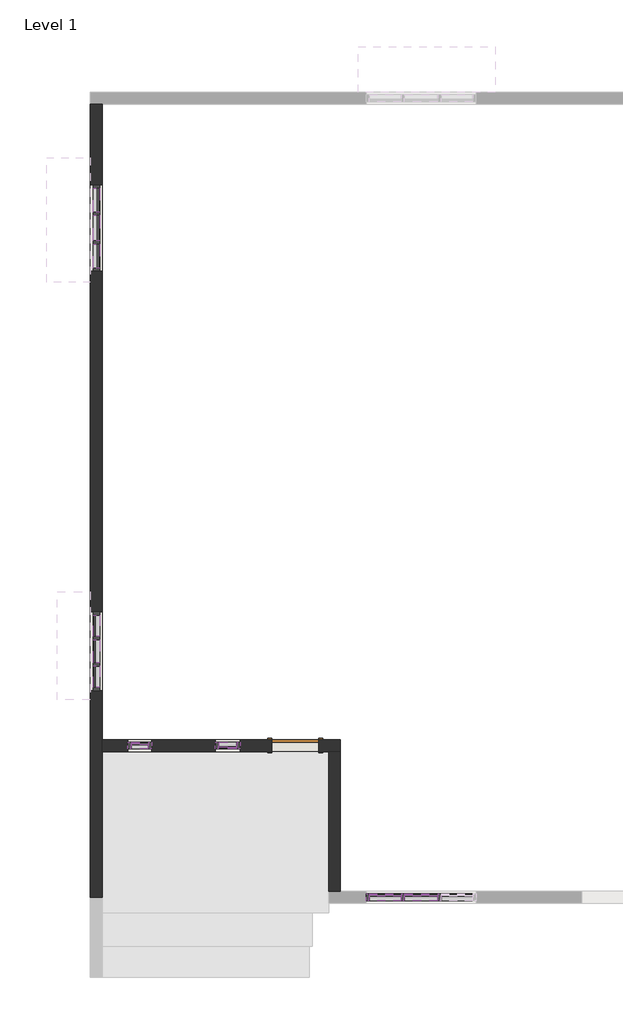
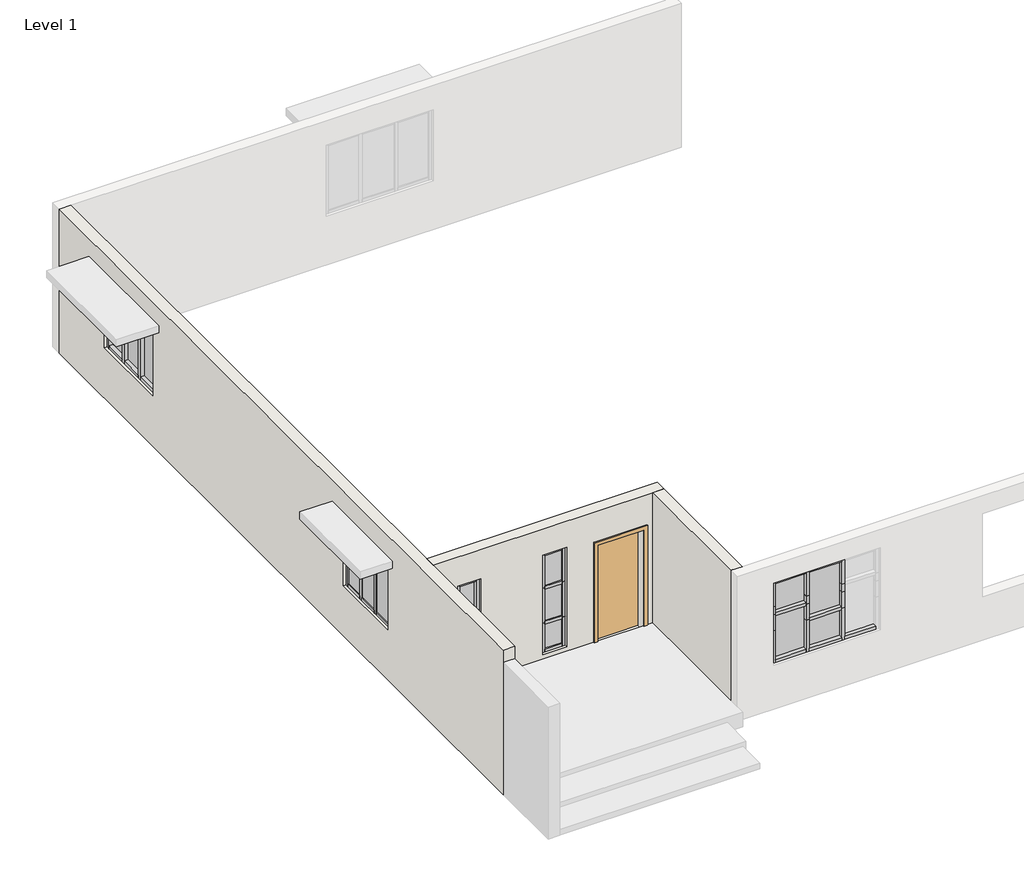
# One storey, part 1 of 2: 59 members, 16 plates, 3 walls, 1 door.
"""IFC4 building model written with IfcOpenShell, lengths in millimetres."""

from ifc_helpers import new_model, si_unit, origin, origin_with_axes, place, context, project, spatial, polyline, outline, extrude, faceted_brep, transform, mapped, element, save
from components import door_0ca8825f, member_be967ef6, member_b3e0441e, member_3f0e0172, member_eeaa8261, member_5215b92c, member_c2e216af, member_baa20d8e, member_e53b78c9, member_4e7e4155, member_f8dc38bf, member_2caf9219, member_d39130fe, member_285f5b4f, member_585e2b51, member_e58ec603, member_e9f63e68, member_ee3d4f96, member_0c1408be, member_ff9f2d30, member_2ebf4a73, member_5535eeb3, member_d9285493, member_ead4612c, member_dc106669, member_bc7dbe04, member_a7a962ec, member_fe78aa24, system_panel_glazed_9fd70c8e, system_panel_glazed_3bdca378, system_panel_glazed_3f50d1a2, system_panel_glazed_776d8ebc, system_panel_glazed_04b6ff1d, system_panel_glazed_0d343f02, system_panel_glazed_5f4e04c5, system_panel_glazed_8b3a0672, system_panel_glazed_8616aaf2, system_panel_glazed_59e6c1d1, system_panel_glazed_1cd5f074, system_panel_glazed_85fa307d, system_panel_glazed_617ab36c

model = new_model("IFC4")

# Units and contexts
model_context = context("Model", 3, world=origin())
ifc_project = project(units=[si_unit("LENGTHUNIT", "METRE", prefix="MILLI")], contexts=[model_context])

# Site, building, storey
site = spatial("IfcSite", under=ifc_project)
building = spatial("IfcBuilding", under=site)
storey = spatial("IfcBuildingStorey", under=building, Name="Level 1", Elevation=0.0)

# Door
placement = place(None, origin())
door_shape = door_0ca8825f(model_context)
element("IfcDoor", 1, ObjectType="Single-Flush : 36\" x 84\"", at=placement, inside=storey, context=model_context, shape_type="MappedRepresentation", body=[
    mapped(door_shape, transform((-17883.2161422, -11856.2171312, 203.2), x_axis=(1.0, 0.0, 0.0), y_axis=(0.0, 1.0, 0.0), z_axis=(0.0, 0.0, 1.0))),
])

# Members
member_shape = member_be967ef6(model_context)
element("IfcMember", 2, ObjectType="Rectangular Mullion : 2.5\" x 5\" rectangular", at=placement, inside=storey, context=model_context, shape_type="MappedRepresentation", body=[
    mapped(member_shape, transform((-16511.6161422, -14789.9171312, 1612.541933), x_axis=(-1.0, 0.0, 0.0), y_axis=(0.0, -1.0, 0.0), z_axis=(0.0, 0.0, 1.0))),
])
member_2_shape = member_b3e0441e(model_context)
element("IfcMember", 3, ObjectType="Rectangular Mullion : 2.5\" x 5\" rectangular", at=placement, inside=storey, context=model_context, shape_type="MappedRepresentation", body=[
    mapped(member_2_shape, transform((-16511.6161422, -14789.9171312, 2663.1790149), x_axis=(-1.0, 0.0, 0.0), y_axis=(0.0, -1.0, 0.0), z_axis=(0.0, 0.0, 1.0))),
])
member_3_shape = member_3f0e0172(model_context)
element("IfcMember", 4, ObjectType="Rectangular Mullion : 2.5\" x 5\" rectangular", at=placement, inside=storey, context=model_context, shape_type="MappedRepresentation", body=[
    mapped(member_3_shape, transform((-15057.4661422, -14789.9171312, 934.5922675), x_axis=(0.0, 0.0, -1.0), y_axis=(0.0, -1.0, 0.0), z_axis=(-1.0, 0.0, 0.0))),
])
element("IfcMember", 5, ObjectType="Rectangular Mullion : 2.5\" x 5\" rectangular", at=placement, inside=storey, context=model_context, shape_type="MappedRepresentation", body=[
    mapped(member_3_shape, transform((-16448.1161422, -14789.9171312, 934.5922675), x_axis=(0.0, 0.0, -1.0), y_axis=(0.0, -1.0, 0.0), z_axis=(-1.0, 0.0, 0.0))),
])
element("IfcMember", 6, ObjectType="Rectangular Mullion : 2.5\" x 5\" rectangular", at=placement, inside=storey, context=model_context, shape_type="MappedRepresentation", body=[
    mapped(member_3_shape, transform((-15832.1661422, -14789.9171312, 2663.1790149), x_axis=(0.0, 0.0, 1.0), y_axis=(0.0, -1.0, 0.0), z_axis=(1.0, 0.0, 0.0))),
])
member_4_shape = member_eeaa8261(model_context)
element("IfcMember", 7, ObjectType="Rectangular Mullion : 2.5\" x 5\" rectangular", at=placement, inside=storey, context=model_context, shape_type="MappedRepresentation", body=[
    mapped(member_4_shape, transform((-15800.4161422, -14789.9171312, 2121.0041821), x_axis=(1.0, 0.0, 0.0), y_axis=(0.0, -1.0, 0.0), z_axis=(0.0, 0.0, -1.0))),
])
member_5_shape = member_5215b92c(model_context)
element("IfcMember", 8, ObjectType="Rectangular Mullion : 2.5\" x 5\" rectangular", at=placement, inside=storey, context=model_context, shape_type="MappedRepresentation", body=[
    mapped(member_5_shape, transform((-15768.6661422, -14789.9171312, 934.5922675), x_axis=(0.0, 0.0, -1.0), y_axis=(0.0, -1.0, 0.0), z_axis=(-1.0, 0.0, 0.0))),
])
element("IfcMember", 9, ObjectType="Rectangular Mullion : 2.5\" x 5\" rectangular", at=placement, inside=storey, context=model_context, shape_type="MappedRepresentation", body=[
    mapped(member_5_shape, transform((-15120.9661422, -14789.9171312, 2663.1790149), x_axis=(0.0, 0.0, 1.0), y_axis=(0.0, -1.0, 0.0), z_axis=(1.0, 0.0, 0.0))),
])
member_6_shape = member_c2e216af(model_context)
element("IfcMember", 10, ObjectType="Rectangular Mullion : 2.5\" x 5\" rectangular", at=placement, inside=storey, context=model_context, shape_type="MappedRepresentation", body=[
    mapped(member_6_shape, transform((-15089.2161422, -14789.9171312, 1612.541933), x_axis=(1.0, 0.0, 0.0), y_axis=(0.0, -1.0, 0.0), z_axis=(0.0, 0.0, -1.0))),
])
member_7_shape = member_baa20d8e(model_context)
element("IfcMember", 11, ObjectType="Rectangular Mullion : 2.5\" x 5\" rectangular", at=placement, inside=storey, context=model_context, shape_type="MappedRepresentation", body=[
    mapped(member_7_shape, transform((-15800.4161422, -14789.9171312, 934.5922675), x_axis=(1.0, 0.0, 0.0), y_axis=(0.0, -1.0, 0.0), z_axis=(0.0, 0.0, -1.0))),
])
element("IfcMember", 12, ObjectType="Rectangular Mullion : 2.5\" x 5\" rectangular", at=placement, inside=storey, context=model_context, shape_type="MappedRepresentation", body=[
    mapped(member_7_shape, transform((-15089.2161422, -14789.9171312, 934.5922675), x_axis=(1.0, 0.0, 0.0), y_axis=(0.0, -1.0, 0.0), z_axis=(0.0, 0.0, -1.0))),
])
member_8_shape = member_e53b78c9(model_context)
element("IfcMember", 13, ObjectType="Rectangular Mullion : 2.5\" x 5\" rectangular", at=placement, inside=storey, context=model_context, shape_type="MappedRepresentation", body=[
    mapped(member_8_shape, transform((-15120.9661422, -14789.9171312, 1612.541933), x_axis=(0.0, 0.0, 1.0), y_axis=(0.0, -1.0, 0.0), z_axis=(1.0, 0.0, 0.0))),
])
element("IfcMember", 14, ObjectType="Rectangular Mullion : 2.5\" x 5\" rectangular", at=placement, inside=storey, context=model_context, shape_type="MappedRepresentation", body=[
    mapped(member_6_shape, transform((-15800.4161422, -14789.9171312, 1612.541933), x_axis=(1.0, 0.0, 0.0), y_axis=(0.0, -1.0, 0.0), z_axis=(0.0, 0.0, -1.0))),
])
member_9_shape = member_4e7e4155(model_context)
element("IfcMember", 15, ObjectType="Rectangular Mullion : 2.5\" x 5\" rectangular", at=placement, inside=storey, context=model_context, shape_type="MappedRepresentation", body=[
    mapped(member_9_shape, transform((-15800.4161422, -14789.9171312, 1951.5167658), x_axis=(1.0, 0.0, 0.0), y_axis=(0.0, -1.0, 0.0), z_axis=(0.0, 0.0, -1.0))),
])
member_10_shape = member_f8dc38bf(model_context)
element("IfcMember", 16, ObjectType="Rectangular Mullion : 2.5\" x 5\" rectangular", at=placement, inside=storey, context=model_context, shape_type="MappedRepresentation", body=[
    mapped(member_10_shape, transform((-15832.1661422, -14789.9171312, 1951.5167658), x_axis=(0.0, 0.0, 1.0), y_axis=(0.0, -1.0, 0.0), z_axis=(1.0, 0.0, 0.0))),
])
member_11_shape = member_2caf9219(model_context)
element("IfcMember", 17, ObjectType="Rectangular Mullion : 2.5\" x 5\" rectangular", at=placement, inside=storey, context=model_context, shape_type="MappedRepresentation", body=[
    mapped(member_11_shape, transform((-16511.6161422, -14789.9171312, 2121.0041821), x_axis=(-1.0, 0.0, 0.0), y_axis=(0.0, -1.0, 0.0), z_axis=(0.0, 0.0, 1.0))),
])
member_12_shape = member_d39130fe(model_context)
element("IfcMember", 18, ObjectType="Rectangular Mullion : 2.5\" x 5\" rectangular", at=placement, inside=storey, context=model_context, shape_type="MappedRepresentation", body=[
    mapped(member_12_shape, transform((-16511.6161422, -14789.9171312, 1951.5167658), x_axis=(-1.0, 0.0, 0.0), y_axis=(0.0, -1.0, 0.0), z_axis=(0.0, 0.0, 1.0))),
])
element("IfcMember", 19, ObjectType="Rectangular Mullion : 2.5\" x 5\" rectangular", at=placement, inside=storey, context=model_context, shape_type="MappedRepresentation", body=[
    mapped(member_4_shape, transform((-15089.2161422, -14789.9171312, 2121.0041821), x_axis=(1.0, 0.0, 0.0), y_axis=(0.0, -1.0, 0.0), z_axis=(0.0, 0.0, -1.0))),
])
element("IfcMember", 20, ObjectType="Rectangular Mullion : 2.5\" x 5\" rectangular", at=placement, inside=storey, context=model_context, shape_type="MappedRepresentation", body=[
    mapped(member_9_shape, transform((-15089.2161422, -14789.9171312, 1951.5167658), x_axis=(1.0, 0.0, 0.0), y_axis=(0.0, -1.0, 0.0), z_axis=(0.0, 0.0, -1.0))),
])
member_13_shape = member_285f5b4f(model_context)
element("IfcMember", 21, ObjectType="Rectangular Mullion : 2.5\" x 5\" rectangular", at=placement, inside=storey, context=model_context, shape_type="MappedRepresentation", body=[
    mapped(member_13_shape, transform((-19362.7661422, -11856.2171312, 2493.7660277), x_axis=(0.0, 0.0, 1.0), y_axis=(0.0, 1.0, 0.0), z_axis=(-1.0, 0.0, 0.0))),
])
element("IfcMember", 22, ObjectType="Rectangular Mullion : 2.5\" x 5\" rectangular", at=placement, inside=storey, context=model_context, shape_type="MappedRepresentation", body=[
    mapped(member_13_shape, transform((-19013.5161422, -11856.2171312, 398.0253718), x_axis=(0.0, 0.0, -1.0), y_axis=(0.0, 1.0, 0.0), z_axis=(1.0, 0.0, 0.0))),
])
member_14_shape = member_585e2b51(model_context)
element("IfcMember", 23, ObjectType="Rectangular Mullion : 2.5\" x 5\" rectangular", at=placement, inside=storey, context=model_context, shape_type="MappedRepresentation", body=[
    mapped(member_14_shape, transform((-19362.7661422, -11856.2171312, 1014.0956997), x_axis=(0.0, 0.0, 1.0), y_axis=(0.0, 1.0, 0.0), z_axis=(-1.0, 0.0, 0.0))),
])
element("IfcMember", 24, ObjectType="Rectangular Mullion : 2.5\" x 5\" rectangular", at=placement, inside=storey, context=model_context, shape_type="MappedRepresentation", body=[
    mapped(member_14_shape, transform((-19362.7661422, -11856.2171312, 1753.9308637), x_axis=(0.0, 0.0, 1.0), y_axis=(0.0, 1.0, 0.0), z_axis=(-1.0, 0.0, 0.0))),
])
member_15_shape = member_e58ec603(model_context)
element("IfcMember", 25, ObjectType="Rectangular Mullion : 2.5\" x 5\" rectangular", at=placement, inside=storey, context=model_context, shape_type="MappedRepresentation", body=[
    mapped(member_15_shape, transform((-19426.2661422, -11856.2171312, 398.0253718), x_axis=(-1.0, 0.0, 0.0), y_axis=(0.0, 1.0, 0.0), z_axis=(0.0, 0.0, -1.0))),
])
element("IfcMember", 26, ObjectType="Rectangular Mullion : 2.5\" x 5\" rectangular", at=placement, inside=storey, context=model_context, shape_type="MappedRepresentation", body=[
    mapped(member_15_shape, transform((-18950.0161422, -11856.2171312, 1014.0956997), x_axis=(1.0, 0.0, 0.0), y_axis=(0.0, 1.0, 0.0), z_axis=(0.0, 0.0, 1.0))),
])
member_16_shape = member_e9f63e68(model_context)
element("IfcMember", 27, ObjectType="Rectangular Mullion : 2.5\" x 5\" rectangular", at=placement, inside=storey, context=model_context, shape_type="MappedRepresentation", body=[
    mapped(member_16_shape, transform((-19426.2661422, -11856.2171312, 1753.9308637), x_axis=(-1.0, 0.0, 0.0), y_axis=(0.0, 1.0, 0.0), z_axis=(0.0, 0.0, -1.0))),
])
element("IfcMember", 28, ObjectType="Rectangular Mullion : 2.5\" x 5\" rectangular", at=placement, inside=storey, context=model_context, shape_type="MappedRepresentation", body=[
    mapped(member_16_shape, transform((-19426.2661422, -11856.2171312, 1014.0956997), x_axis=(-1.0, 0.0, 0.0), y_axis=(0.0, 1.0, 0.0), z_axis=(0.0, 0.0, -1.0))),
])
element("IfcMember", 29, ObjectType="Rectangular Mullion : 2.5\" x 5\" rectangular", at=placement, inside=storey, context=model_context, shape_type="MappedRepresentation", body=[
    mapped(member_16_shape, transform((-18950.0161422, -11856.2171312, 1753.9308637), x_axis=(1.0, 0.0, 0.0), y_axis=(0.0, 1.0, 0.0), z_axis=(0.0, 0.0, 1.0))),
])
element("IfcMember", 30, ObjectType="Rectangular Mullion : 2.5\" x 5\" rectangular", at=placement, inside=storey, context=model_context, shape_type="MappedRepresentation", body=[
    mapped(member_16_shape, transform((-18950.0161422, -11856.2171312, 2493.7660277), x_axis=(1.0, 0.0, 0.0), y_axis=(0.0, 1.0, 0.0), z_axis=(0.0, 0.0, 1.0))),
])
member_17_shape = member_ee3d4f96(model_context)
element("IfcMember", 31, ObjectType="Rectangular Mullion : 2.5\" x 5\" rectangular", at=placement, inside=storey, context=model_context, shape_type="MappedRepresentation", body=[
    mapped(member_17_shape, transform((-21121.7161422, -11856.2171312, 1065.8254734), x_axis=(-1.0, 0.0, 0.0), y_axis=(0.0, -1.0, 0.0), z_axis=(0.0, 0.0, 1.0))),
])
element("IfcMember", 32, ObjectType="Rectangular Mullion : 2.5\" x 5\" rectangular", at=placement, inside=storey, context=model_context, shape_type="MappedRepresentation", body=[
    mapped(member_17_shape, transform((-21121.7161422, -11856.2171312, 1750.6277467), x_axis=(-1.0, 0.0, 0.0), y_axis=(0.0, -1.0, 0.0), z_axis=(0.0, 0.0, 1.0))),
])
element("IfcMember", 33, ObjectType="Rectangular Mullion : 2.5\" x 5\" rectangular", at=placement, inside=storey, context=model_context, shape_type="MappedRepresentation", body=[
    mapped(member_17_shape, transform((-21121.7161422, -11856.2171312, 2435.43002), x_axis=(-1.0, 0.0, 0.0), y_axis=(0.0, -1.0, 0.0), z_axis=(0.0, 0.0, 1.0))),
])
member_18_shape = member_0c1408be(model_context)
element("IfcMember", 34, ObjectType="Rectangular Mullion : 2.5\" x 5\" rectangular", at=placement, inside=storey, context=model_context, shape_type="MappedRepresentation", body=[
    mapped(member_18_shape, transform((-20728.0161422, -11856.2171312, 1750.6277467), x_axis=(0.0, 0.0, 1.0), y_axis=(0.0, -1.0, 0.0), z_axis=(1.0, 0.0, 0.0))),
])
element("IfcMember", 35, ObjectType="Rectangular Mullion : 2.5\" x 5\" rectangular", at=placement, inside=storey, context=model_context, shape_type="MappedRepresentation", body=[
    mapped(member_18_shape, transform((-20728.0161422, -11856.2171312, 1065.8254734), x_axis=(0.0, 0.0, 1.0), y_axis=(0.0, -1.0, 0.0), z_axis=(1.0, 0.0, 0.0))),
])
member_19_shape = member_ff9f2d30(model_context)
element("IfcMember", 36, ObjectType="Rectangular Mullion : 2.5\" x 5\" rectangular", at=placement, inside=storey, context=model_context, shape_type="MappedRepresentation", body=[
    mapped(member_19_shape, transform((-21058.2161422, -11856.2171312, 381.0232001), x_axis=(0.0, 0.0, -1.0), y_axis=(0.0, -1.0, 0.0), z_axis=(-1.0, 0.0, 0.0))),
])
element("IfcMember", 37, ObjectType="Rectangular Mullion : 2.5\" x 5\" rectangular", at=placement, inside=storey, context=model_context, shape_type="MappedRepresentation", body=[
    mapped(member_19_shape, transform((-20728.0161422, -11856.2171312, 2435.43002), x_axis=(0.0, 0.0, 1.0), y_axis=(0.0, -1.0, 0.0), z_axis=(1.0, 0.0, 0.0))),
])
element("IfcMember", 38, ObjectType="Rectangular Mullion : 2.5\" x 5\" rectangular", at=placement, inside=storey, context=model_context, shape_type="MappedRepresentation", body=[
    mapped(member_17_shape, transform((-20664.5161422, -11856.2171312, 1065.8254734), x_axis=(1.0, 0.0, 0.0), y_axis=(0.0, -1.0, 0.0), z_axis=(0.0, 0.0, -1.0))),
])
element("IfcMember", 39, ObjectType="Rectangular Mullion : 2.5\" x 5\" rectangular", at=placement, inside=storey, context=model_context, shape_type="MappedRepresentation", body=[
    mapped(member_17_shape, transform((-20664.5161422, -11856.2171312, 1750.6277467), x_axis=(1.0, 0.0, 0.0), y_axis=(0.0, -1.0, 0.0), z_axis=(0.0, 0.0, -1.0))),
])
element("IfcMember", 40, ObjectType="Rectangular Mullion : 2.5\" x 5\" rectangular", at=placement, inside=storey, context=model_context, shape_type="MappedRepresentation", body=[
    mapped(member_17_shape, transform((-20664.5161422, -11856.2171312, 381.0232001), x_axis=(1.0, 0.0, 0.0), y_axis=(0.0, -1.0, 0.0), z_axis=(0.0, 0.0, -1.0))),
])
member_20_shape = member_2ebf4a73(model_context)
element("IfcMember", 41, ObjectType="Rectangular Mullion : 2.5\" x 5\" rectangular", at=placement, inside=storey, context=model_context, shape_type="MappedRepresentation", body=[
    mapped(member_20_shape, transform((-21731.3161422, -2083.5671312, 2524.5687713), x_axis=(0.0, 0.0, 1.0), y_axis=(-1.0, 0.0, 0.0), z_axis=(0.0, -1.0, 0.0))),
])
member_21_shape = member_5535eeb3(model_context)
element("IfcMember", 42, ObjectType="Rectangular Mullion : 2.5\" x 5\" rectangular", at=placement, inside=storey, context=model_context, shape_type="MappedRepresentation", body=[
    mapped(member_21_shape, transform((-21731.3161422, -1524.7671312, 2524.5687713), x_axis=(0.0, 0.0, 1.0), y_axis=(-1.0, 0.0, 0.0), z_axis=(0.0, -1.0, 0.0))),
])
element("IfcMember", 43, ObjectType="Rectangular Mullion : 2.5\" x 5\" rectangular", at=placement, inside=storey, context=model_context, shape_type="MappedRepresentation", body=[
    mapped(member_21_shape, transform((-21731.3161422, -2610.6171312, 2524.5687713), x_axis=(0.0, 0.0, 1.0), y_axis=(-1.0, 0.0, 0.0), z_axis=(0.0, -1.0, 0.0))),
])
member_22_shape = member_d9285493(model_context)
element("IfcMember", 44, ObjectType="Rectangular Mullion : 2.5\" x 5\" rectangular", at=placement, inside=storey, context=model_context, shape_type="MappedRepresentation", body=[
    mapped(member_22_shape, transform((-21731.3161422, -1556.5171312, 1066.8702548), x_axis=(0.0, -1.0, 0.0), y_axis=(-1.0, 0.0, 0.0), z_axis=(0.0, 0.0, -1.0))),
])
element("IfcMember", 45, ObjectType="Rectangular Mullion : 2.5\" x 5\" rectangular", at=placement, inside=storey, context=model_context, shape_type="MappedRepresentation", body=[
    mapped(member_22_shape, transform((-21731.3161422, -2115.3171312, 1066.8702548), x_axis=(0.0, -1.0, 0.0), y_axis=(-1.0, 0.0, 0.0), z_axis=(0.0, 0.0, -1.0))),
])
element("IfcMember", 46, ObjectType="Rectangular Mullion : 2.5\" x 5\" rectangular", at=placement, inside=storey, context=model_context, shape_type="MappedRepresentation", body=[
    mapped(member_20_shape, transform((-21731.3161422, -1588.2671312, 1066.8702548), x_axis=(0.0, 0.0, -1.0), y_axis=(-1.0, 0.0, 0.0), z_axis=(0.0, 1.0, 0.0))),
])
element("IfcMember", 47, ObjectType="Rectangular Mullion : 2.5\" x 5\" rectangular", at=placement, inside=storey, context=model_context, shape_type="MappedRepresentation", body=[
    mapped(member_21_shape, transform((-21731.3161422, -2147.0671312, 1066.8702548), x_axis=(0.0, 0.0, -1.0), y_axis=(-1.0, 0.0, 0.0), z_axis=(0.0, 1.0, 0.0))),
])
element("IfcMember", 48, ObjectType="Rectangular Mullion : 2.5\" x 5\" rectangular", at=placement, inside=storey, context=model_context, shape_type="MappedRepresentation", body=[
    mapped(member_21_shape, transform((-21731.3161422, -1061.2171312, 1066.8702548), x_axis=(0.0, 0.0, -1.0), y_axis=(-1.0, 0.0, 0.0), z_axis=(0.0, 1.0, 0.0))),
])
member_23_shape = member_ead4612c(model_context)
element("IfcMember", 49, ObjectType="Rectangular Mullion : 2.5\" x 5\" rectangular", at=placement, inside=storey, context=model_context, shape_type="MappedRepresentation", body=[
    mapped(member_23_shape, transform((-21731.3161422, -997.7171312, 2524.5687713), x_axis=(0.0, 1.0, 0.0), y_axis=(-1.0, 0.0, 0.0), z_axis=(0.0, 0.0, 1.0))),
])
element("IfcMember", 50, ObjectType="Rectangular Mullion : 2.5\" x 5\" rectangular", at=placement, inside=storey, context=model_context, shape_type="MappedRepresentation", body=[
    mapped(member_23_shape, transform((-21731.3161422, -2674.1171312, 1066.8702548), x_axis=(0.0, -1.0, 0.0), y_axis=(-1.0, 0.0, 0.0), z_axis=(0.0, 0.0, -1.0))),
])
member_24_shape = member_dc106669(model_context)
element("IfcMember", 51, ObjectType="Rectangular Mullion : 2.5\" x 5\" rectangular", at=placement, inside=storey, context=model_context, shape_type="MappedRepresentation", body=[
    mapped(member_24_shape, transform((-21731.3161422, -10313.1671312, 2454.0538094), x_axis=(0.0, 0.0, 1.0), y_axis=(1.0, 0.0, 0.0), z_axis=(0.0, 1.0, 0.0))),
])
element("IfcMember", 52, ObjectType="Rectangular Mullion : 2.5\" x 5\" rectangular", at=placement, inside=storey, context=model_context, shape_type="MappedRepresentation", body=[
    mapped(member_24_shape, transform((-21731.3161422, -9328.9171312, 2454.0538094), x_axis=(0.0, 0.0, 1.0), y_axis=(1.0, 0.0, 0.0), z_axis=(0.0, 1.0, 0.0))),
])
member_25_shape = member_bc7dbe04(model_context)
element("IfcMember", 53, ObjectType="Rectangular Mullion : 2.5\" x 5\" rectangular", at=placement, inside=storey, context=model_context, shape_type="MappedRepresentation", body=[
    mapped(member_25_shape, transform((-21731.3161422, -9805.1671312, 2454.0538094), x_axis=(0.0, 0.0, 1.0), y_axis=(1.0, 0.0, 0.0), z_axis=(0.0, 1.0, 0.0))),
])
member_26_shape = member_a7a962ec(model_context)
element("IfcMember", 54, ObjectType="Rectangular Mullion : 2.5\" x 5\" rectangular", at=placement, inside=storey, context=model_context, shape_type="MappedRepresentation", body=[
    mapped(member_26_shape, transform((-21731.3161422, -9773.4171312, 1052.4206205), x_axis=(0.0, 1.0, 0.0), y_axis=(1.0, 0.0, 0.0), z_axis=(0.0, 0.0, -1.0))),
])
element("IfcMember", 55, ObjectType="Rectangular Mullion : 2.5\" x 5\" rectangular", at=placement, inside=storey, context=model_context, shape_type="MappedRepresentation", body=[
    mapped(member_26_shape, transform((-21731.3161422, -10281.4171312, 1052.4206205), x_axis=(0.0, 1.0, 0.0), y_axis=(1.0, 0.0, 0.0), z_axis=(0.0, 0.0, -1.0))),
])
element("IfcMember", 56, ObjectType="Rectangular Mullion : 2.5\" x 5\" rectangular", at=placement, inside=storey, context=model_context, shape_type="MappedRepresentation", body=[
    mapped(member_25_shape, transform((-21731.3161422, -10249.6671312, 1052.4206205), x_axis=(0.0, 0.0, -1.0), y_axis=(1.0, 0.0, 0.0), z_axis=(0.0, -1.0, 0.0))),
])
element("IfcMember", 57, ObjectType="Rectangular Mullion : 2.5\" x 5\" rectangular", at=placement, inside=storey, context=model_context, shape_type="MappedRepresentation", body=[
    mapped(member_24_shape, transform((-21731.3161422, -9741.6671312, 1052.4206205), x_axis=(0.0, 0.0, -1.0), y_axis=(1.0, 0.0, 0.0), z_axis=(0.0, -1.0, 0.0))),
])
element("IfcMember", 58, ObjectType="Rectangular Mullion : 2.5\" x 5\" rectangular", at=placement, inside=storey, context=model_context, shape_type="MappedRepresentation", body=[
    mapped(member_24_shape, transform((-21731.3161422, -10725.9171312, 1052.4206205), x_axis=(0.0, 0.0, -1.0), y_axis=(1.0, 0.0, 0.0), z_axis=(0.0, -1.0, 0.0))),
])
member_27_shape = member_fe78aa24(model_context)
element("IfcMember", 59, ObjectType="Rectangular Mullion : 2.5\" x 5\" rectangular", at=placement, inside=storey, context=model_context, shape_type="MappedRepresentation", body=[
    mapped(member_27_shape, transform((-21731.3161422, -10789.4171312, 2454.0538094), x_axis=(0.0, -1.0, 0.0), y_axis=(1.0, 0.0, 0.0), z_axis=(0.0, 0.0, 1.0))),
])
element("IfcMember", 60, ObjectType="Rectangular Mullion : 2.5\" x 5\" rectangular", at=placement, inside=storey, context=model_context, shape_type="MappedRepresentation", body=[
    mapped(member_27_shape, transform((-21731.3161422, -9265.4171312, 1052.4206205), x_axis=(0.0, 1.0, 0.0), y_axis=(1.0, 0.0, 0.0), z_axis=(0.0, 0.0, -1.0))),
])

# Plates
system_panel_glazed_shape = system_panel_glazed_9fd70c8e(model_context)
element("IfcPlate", 61, ObjectType="System Panel : Glazed", at=placement, inside=storey, context=model_context, shape_type="MappedRepresentation", body=[
    mapped(system_panel_glazed_shape, transform((-15444.8161422, -14789.9171312, 998.0922675), x_axis=(1.0, 0.0, 0.0), y_axis=(0.0, 1.0, 0.0), z_axis=(0.0, 0.0, 1.0))),
])
system_panel_glazed_2_shape = system_panel_glazed_3bdca378(model_context)
element("IfcPlate", 62, ObjectType="System Panel : Glazed", at=placement, inside=storey, context=model_context, shape_type="MappedRepresentation", body=[
    mapped(system_panel_glazed_2_shape, transform((-15444.8161422, -14789.9171312, 1644.291933), x_axis=(1.0, 0.0, 0.0), y_axis=(0.0, 1.0, 0.0), z_axis=(0.0, 0.0, 1.0))),
])
system_panel_glazed_3_shape = system_panel_glazed_3f50d1a2(model_context)
element("IfcPlate", 63, ObjectType="System Panel : Glazed", at=placement, inside=storey, context=model_context, shape_type="MappedRepresentation", body=[
    mapped(system_panel_glazed_3_shape, transform((-16140.1411422, -14789.9171312, 998.0922675), x_axis=(1.0, 0.0, 0.0), y_axis=(0.0, 1.0, 0.0), z_axis=(0.0, 0.0, 1.0))),
])
system_panel_glazed_4_shape = system_panel_glazed_776d8ebc(model_context)
element("IfcPlate", 64, ObjectType="System Panel : Glazed", at=placement, inside=storey, context=model_context, shape_type="MappedRepresentation", body=[
    mapped(system_panel_glazed_4_shape, transform((-16140.1411422, -14789.9171312, 1983.2667658), x_axis=(1.0, 0.0, 0.0), y_axis=(0.0, 1.0, 0.0), z_axis=(0.0, 0.0, 1.0))),
])
system_panel_glazed_5_shape = system_panel_glazed_04b6ff1d(model_context)
element("IfcPlate", 65, ObjectType="System Panel : Glazed", at=placement, inside=storey, context=model_context, shape_type="MappedRepresentation", body=[
    mapped(system_panel_glazed_5_shape, transform((-19188.1411422, -11856.2171312, 1045.8456997), x_axis=(-1.0, 0.0, 0.0), y_axis=(0.0, -1.0, 0.0), z_axis=(0.0, 0.0, 1.0))),
])
system_panel_glazed_6_shape = system_panel_glazed_0d343f02(model_context)
element("IfcPlate", 66, ObjectType="System Panel : Glazed", at=placement, inside=storey, context=model_context, shape_type="MappedRepresentation", body=[
    mapped(system_panel_glazed_6_shape, transform((-19188.1411422, -11856.2171312, 461.5253718), x_axis=(-1.0, 0.0, 0.0), y_axis=(0.0, -1.0, 0.0), z_axis=(0.0, 0.0, 1.0))),
])
system_panel_glazed_7_shape = system_panel_glazed_5f4e04c5(model_context)
element("IfcPlate", 67, ObjectType="System Panel : Glazed", at=placement, inside=storey, context=model_context, shape_type="MappedRepresentation", body=[
    mapped(system_panel_glazed_7_shape, transform((-19188.1411422, -11856.2171312, 1785.6808637), x_axis=(-1.0, 0.0, 0.0), y_axis=(0.0, -1.0, 0.0), z_axis=(0.0, 0.0, 1.0))),
])
system_panel_glazed_8_shape = system_panel_glazed_8b3a0672(model_context)
element("IfcPlate", 68, ObjectType="System Panel : Glazed", at=placement, inside=storey, context=model_context, shape_type="MappedRepresentation", body=[
    mapped(system_panel_glazed_8_shape, transform((-20893.1161422, -11856.2171312, 444.5232001), x_axis=(1.0, 0.0, 0.0), y_axis=(0.0, 1.0, 0.0), z_axis=(0.0, 0.0, 1.0))),
])
element("IfcPlate", 69, ObjectType="System Panel : Glazed", at=placement, inside=storey, context=model_context, shape_type="MappedRepresentation", body=[
    mapped(system_panel_glazed_8_shape, transform((-20893.1161422, -11856.2171312, 1782.3777467), x_axis=(1.0, 0.0, 0.0), y_axis=(0.0, 1.0, 0.0), z_axis=(0.0, 0.0, 1.0))),
])
system_panel_glazed_9_shape = system_panel_glazed_8616aaf2(model_context)
element("IfcPlate", 70, ObjectType="System Panel : Glazed", at=placement, inside=storey, context=model_context, shape_type="MappedRepresentation", body=[
    mapped(system_panel_glazed_9_shape, transform((-20893.1161422, -11856.2171312, 1097.5754734), x_axis=(1.0, 0.0, 0.0), y_axis=(0.0, 1.0, 0.0), z_axis=(0.0, 0.0, 1.0))),
])
system_panel_glazed_10_shape = system_panel_glazed_59e6c1d1(model_context)
element("IfcPlate", 71, ObjectType="System Panel : Glazed", at=placement, inside=storey, context=model_context, shape_type="MappedRepresentation", body=[
    mapped(system_panel_glazed_10_shape, transform((-21731.3161422, -1292.9921312, 1130.3702548), x_axis=(0.0, -1.0, 0.0), y_axis=(1.0, 0.0, 0.0), z_axis=(0.0, 0.0, 1.0))),
])
element("IfcPlate", 72, ObjectType="System Panel : Glazed", at=placement, inside=storey, context=model_context, shape_type="MappedRepresentation", body=[
    mapped(system_panel_glazed_10_shape, transform((-21731.3161422, -2378.8421312, 1130.3702548), x_axis=(0.0, -1.0, 0.0), y_axis=(1.0, 0.0, 0.0), z_axis=(0.0, 0.0, 1.0))),
])
system_panel_glazed_11_shape = system_panel_glazed_1cd5f074(model_context)
element("IfcPlate", 73, ObjectType="System Panel : Glazed", at=placement, inside=storey, context=model_context, shape_type="MappedRepresentation", body=[
    mapped(system_panel_glazed_11_shape, transform((-21731.3161422, -1835.9171312, 1130.3702548), x_axis=(0.0, -1.0, 0.0), y_axis=(1.0, 0.0, 0.0), z_axis=(0.0, 0.0, 1.0))),
])
system_panel_glazed_12_shape = system_panel_glazed_85fa307d(model_context)
element("IfcPlate", 74, ObjectType="System Panel : Glazed", at=placement, inside=storey, context=model_context, shape_type="MappedRepresentation", body=[
    mapped(system_panel_glazed_12_shape, transform((-21731.3161422, -10519.5421312, 1115.9206205), x_axis=(0.0, 1.0, 0.0), y_axis=(-1.0, 0.0, 0.0), z_axis=(0.0, 0.0, 1.0))),
])
element("IfcPlate", 75, ObjectType="System Panel : Glazed", at=placement, inside=storey, context=model_context, shape_type="MappedRepresentation", body=[
    mapped(system_panel_glazed_12_shape, transform((-21731.3161422, -9535.2921312, 1115.9206205), x_axis=(0.0, 1.0, 0.0), y_axis=(-1.0, 0.0, 0.0), z_axis=(0.0, 0.0, 1.0))),
])
system_panel_glazed_13_shape = system_panel_glazed_617ab36c(model_context)
element("IfcPlate", 76, ObjectType="System Panel : Glazed", at=placement, inside=storey, context=model_context, shape_type="MappedRepresentation", body=[
    mapped(system_panel_glazed_13_shape, transform((-21731.3161422, -10027.4171312, 1115.9206205), x_axis=(0.0, 1.0, 0.0), y_axis=(-1.0, 0.0, 0.0), z_axis=(0.0, 0.0, 1.0))),
])

# Walls
element("IfcWall", 77, ObjectType="9\"", at=placement, inside=storey, context=model_context, shape_type="Brep", body=[
    faceted_brep([(-21845.6161422, 564.3828688, 0.0), (-21845.6161422, -14789.9171312, 0.0), (-21845.6161422, -14789.9171312, 3048.0), (-21845.6161422, 564.3828688, 3048.0), (-21845.6161422, -997.7171312, 1066.8702548), (-21845.6161422, -997.7171312, 2524.5687713), (-21845.6161422, -2674.1171312, 2524.5687713), (-21845.6161422, -2674.1171312, 1066.8702548), (-21845.6161422, -10789.4171312, 2454.0538094), (-21845.6161422, -10789.4171312, 1052.4206205), (-21845.6161422, -9265.4171312, 1052.4206205), (-21845.6161422, -9265.4171312, 2454.0538094), (-21617.0161422, -14789.9171312, 0.0), (-21617.0161422, -11970.5171312, 0.0), (-21617.0161422, -11741.9171312, 0.0), (-21617.0161422, 564.3828688, 0.0), (-21617.0161422, 564.3828688, 3048.0), (-21617.0161422, -11741.9171312, 3048.0), (-21617.0161422, -11970.5171312, 3048.0), (-21617.0161422, -14789.9171312, 3048.0), (-21617.0161422, -997.7171312, 2524.5687713), (-21617.0161422, -997.7171312, 1066.8702548), (-21617.0161422, -2674.1171312, 1066.8702548), (-21617.0161422, -2674.1171312, 2524.5687713), (-21617.0161422, -10789.4171312, 1052.4206205), (-21617.0161422, -10789.4171312, 2454.0538094), (-21617.0161422, -9265.4171312, 2454.0538094), (-21617.0161422, -9265.4171312, 1052.4206205)], [[[0, 1, 2, 3], [4, 5, 6, 7], [8, 9, 10, 11]], [[12, 13, 14, 15, 16, 17, 18, 19], [20, 21, 22, 23], [24, 25, 26, 27]], [[1, 0, 15, 14, 13, 12]], [[2, 1, 12, 19]], [[3, 2, 19, 18, 17, 16]], [[0, 3, 16, 15]], [[4, 21, 20, 5]], [[5, 20, 23, 6]], [[6, 23, 22, 7]], [[21, 4, 7, 22]], [[24, 9, 8, 25]], [[25, 8, 11, 26]], [[10, 27, 26, 11]], [[9, 24, 27, 10]]]),
])
element("IfcWall", 78, ObjectType="9\"", at=placement, inside=storey, context=model_context, shape_type="Brep", body=[
    faceted_brep([(-21617.0161422, -11970.5171312, 0.0), (-17235.5161422, -11970.5171312, 0.0), (-17006.9161422, -11970.5171312, 0.0), (-17006.9161422, -11970.5171312, 3048.0), (-17235.5161422, -11970.5171312, 3048.0), (-21617.0161422, -11970.5171312, 3048.0), (-17426.0161422, -11970.5171312, 203.2), (-18340.4161422, -11970.5171312, 203.2), (-18340.4161422, -11970.5171312, 2336.8), (-17426.0161422, -11970.5171312, 2336.8), (-18950.0161422, -11970.5171312, 2493.7660277), (-18950.0161422, -11970.5171312, 398.0253718), (-19426.2661422, -11970.5171312, 398.0253718), (-19426.2661422, -11970.5171312, 2493.7660277), (-21121.7161422, -11970.5171312, 381.0232001), (-21121.7161422, -11970.5171312, 2435.43002), (-20664.5161422, -11970.5171312, 2435.43002), (-20664.5161422, -11970.5171312, 381.0232001), (-17006.9161422, -11741.9171312, 0.0), (-21617.0161422, -11741.9171312, 0.0), (-21617.0161422, -11741.9171312, 3048.0), (-17006.9161422, -11741.9171312, 3048.0), (-18340.4161422, -11741.9171312, 203.2), (-17426.0161422, -11741.9171312, 203.2), (-17426.0161422, -11741.9171312, 2336.8), (-18340.4161422, -11741.9171312, 2336.8), (-18950.0161422, -11741.9171312, 398.0253718), (-18950.0161422, -11741.9171312, 2493.7660277), (-19426.2661422, -11741.9171312, 2493.7660277), (-19426.2661422, -11741.9171312, 398.0253718), (-21121.7161422, -11741.9171312, 2435.43002), (-21121.7161422, -11741.9171312, 381.0232001), (-20664.5161422, -11741.9171312, 381.0232001), (-20664.5161422, -11741.9171312, 2435.43002)], [[[0, 1, 2, 3, 4, 5], [6, 7, 8, 9], [10, 11, 12, 13], [14, 15, 16, 17]], [[18, 19, 20, 21], [22, 23, 24, 25], [26, 27, 28, 29], [30, 31, 32, 33]], [[0, 5, 20, 19]], [[3, 2, 18, 21]], [[23, 22, 7, 6]], [[24, 23, 6, 9]], [[25, 24, 9, 8]], [[22, 25, 8, 7]], [[26, 11, 10, 27]], [[27, 10, 13, 28]], [[28, 13, 12, 29]], [[11, 26, 29, 12]], [[30, 15, 14, 31]], [[15, 30, 33, 16]], [[16, 33, 32, 17]], [[31, 14, 17, 32]], [[2, 1, 0, 19, 18]], [[5, 4, 3, 21, 20]]]),
])
element("IfcWall", 79, ObjectType="9\"", at=placement, inside=storey, context=model_context, shape_type="SweptSolid", body=[
    extrude(outline(polyline([(-17235.5161422, -14675.6171312), (-17235.5161422, -11970.5171312), (-17006.9161422, -11970.5171312), (-17006.9161422, -14675.6171312), (-17235.5161422, -14675.6171312)])), origin_with_axes(), (0.0, 0.0, 1.0), 3048.0),
])

save(model, "model.ifc")

# Revit data of these elements
# Type "Single-Flush : 36\" x 84\""
#   Type Mark = "1"
#   Construction Type Id = "MDOOR"
#   Assembly Code = "C1020"
#   Analytic Construction = "Metal"
#   Thickness = 0' - 2"
#   Heat Transfer Coefficient (U) = 0.651978 BTU/(h·ft²·°F)
#   Height = 7' - 0"
#   Trim Projection Ext = 0' - 1"
#   Trim Projection Int = 0' - 1"
#   Trim Width = 0' - 3"
#   Width = 3' - 0"
#   Define Thermal Properties by = 1
#   Define Thermal Properties by = 1
#   Door Material = Door - Panel
#   Frame Material = Door - Frame
#   Visual Light Transmittance = 0
#   Solar Heat Gain Coefficient = 0
#   Function = (empty or 0)
#   Wall Closure = (empty or 0)
# Type "Rectangular Mullion : 2.5\" x 5\" rectangular"
#   built-in parameter 1007304 = 0.416667 (stored number, unit not read)
#   built-in parameter 1007301 = 0.104167 (stored number, unit not read)
#   built-in parameter 1007300 = 0.104167 (stored number, unit not read)
# Type "System Panel : Glazed"
#   Construction Type Id = "GSP4R"
#   Analytic Construction = "1/8 in Pilkington single glazing"
#   Visual Light Transmittance = 0.9
#   Solar Heat Gain Coefficient = 0.86
#   Heat Transfer Coefficient (U) = 1.18115 BTU/(h·ft²·°F)
#   Define Thermal Properties by = 1
# Type "9\""
#   Assembly Code = "B2010"
#   Layers, outside or top first: 0' - 9" no material (function 1)
# Element 1 (IfcDoor, "Single-Flush : 36\" x 84\"")
#   Phase Created = New Construction
#   Materials on its faces: "Door - Frame", "Door - Panel"
# Elements 2, 3, 4, 5, 6, 7, 8, 9, 10, 11, 12, 13, 14, 15, 16, 17, 18, 19, 20, 21, 22, 23, 24, 25, 26, 27, 28, 29, 30, 31, 32, 33, 34, 35, 36, 37, 38, 39, 40, 41, 42, 43, 44, 45, 46, 47, 48, 49, 50, 51, 52, 53, 54, 55, 56, 57, 58, 59, 60 (IfcMember, "Rectangular Mullion : 2.5\" x 5\" rectangular")
#   Phase Created = New Construction
#   Materials on its faces: "Aluminum"
# Elements 61, 62, 63, 64, 65, 66, 67, 68, 69, 70, 71, 72, 73, 74, 75, 76 (IfcPlate, "System Panel : Glazed")
#   Phase Created = New Construction
#   Materials on its faces: "Glass"
# Elements 77, 78, 79 (IfcWall, "9\"")
#   Top Offset = 0' - 0"
#   Base Offset = 0' - 0"
#   Unconnected Height = 10' - 0"
#   wall height = 10' - 0"
#   Phase Created = New Construction
#   Base Constraint = Level 1
#   Materials on its faces: "Default Wall"
# Materials
#   "Door - Panel": class "Wood", colour RGB 210 159 95, transparency 0, Cost = 0
#   "Door - Frame": colour RGB 118 70 51, transparency 0, Cost = 0
#   "Aluminum": class "Metal", colour RGB 247 247 247, transparency 0, Description = "Aluminum 6061", Cost = 0
#   "Glass": class "Glass", colour RGB 0 128 192, transparency 0.75, Description = "Soda Lime Glass", Cost = 0
#   "Default Wall": colour RGB 128 128 128, transparency 0, Cost = 0
